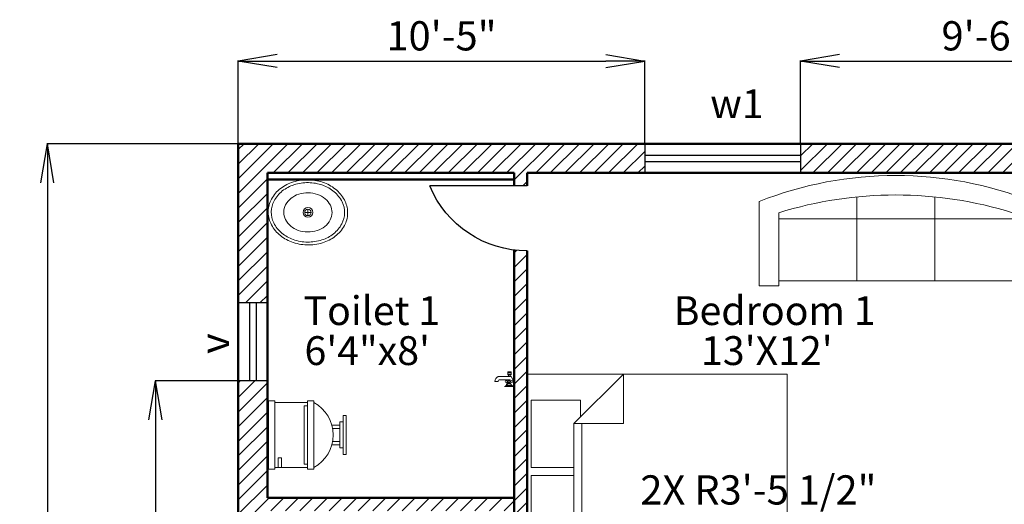
# Model space of a CAD drawing. Units: inches. Extents: x 1856 to 3350, y 1624 to 2224.
# Tile 2 of 7: x 1856 to 2159, y 2016 to 2165. Entities that reach past the tile are written whole.
import ezdxf

# ---------------------------------------------------------------- set-up
doc = ezdxf.new("R2010")
doc.units = ezdxf.units.IN
for name, color, linetype, lineweight in [('A-ANNO-DIMS', 2, 'Continuous', 18), ('A-ANNO-TEXT', 7, 'Continuous', 18), ('A-AREA-IDEN', 7, 'Continuous', 25), ('A-DOOR', 3, 'Continuous', 25), ('A-FLOR-FIXT', 3, 'Continuous', 18), ('A-FURN', 3, 'Continuous', 18), ('A-WALL', 7, 'Continuous', 50), ('A-WALL-PATT', 8, 'Continuous', 13), ('ventilator', 6, 'Continuous', 25), ('window', 4, 'Continuous', 25)]:
    doc.layers.add(name, color=color, linetype=linetype, lineweight=lineweight)
doc.styles.get("Standard").update_dxf_attribs({"font": 'arial.ttf'})
doc.dimstyles.new('ISO-25', dxfattribs={"dimtxt": 9, "dimasz": 12, "dimexe": 0.125, "dimexo": 0.125, "dimgap": 2, "dimtad": 1, "dimtih": 1, "dimtoh": 1, "dimdec": 1, "dimzin": 11, "dimlunit": 4, "dimtxsty": 'Standard', "dimblk": 'OPEN', "dimcen": -0.125, "dimadec": 0, "dimazin": 0, "dimtfac": 1, "dimtdec": 1, "dimtmove": 0, "dimatfit": 3, "dimfxl": 1, "dimarcsym": 0})

# ---------------------------------------------------------------- blocks, each defined once
blk = doc.blocks.new('_Open')
at = {"color": 0, "linetype": 'ByBlock', "lineweight": -2}
for p, q in [((-1, 0.167), (0, 0)), ((-1, -0.167), (0, 0)), ((0, 0), (-1, 0))]:
    blk.add_line(p, q, dxfattribs=at)
blk = doc.blocks.new('*D4')
at = {"layer": 'A-ANNO-DIMS', "color": 0, "lineweight": -2, "transparency": 16777216}
for p, q in [((1922.99, 2126.99), (1864.24, 2126.99)), ((1864.36, 2114.99), (1864.36, 1983.59)), ((1864.36, 1838.99), (1864.36, 1970.4)), ((1922.99, 1826.99), (1864.24, 1826.99))]:
    blk.add_line(p, q, dxfattribs=at)
at = {"layer": 'Defpoints', "color": 0, "transparency": 16777216}
for p in [(1923.11, 2126.99), (1864.36, 1826.99), (1923.11, 1826.99)]:
    blk.add_point(p, dxfattribs=at)
at = {"layer": 'A-ANNO-DIMS', "color": 0, "lineweight": -2, "transparency": 16777216, "xscale": 12, "yscale": 12, "zscale": 12}
for p, rotation in [((1864.36, 2126.99), 90), ((1864.36, 1826.99), 270)]:
    blk.add_blockref('_Open', p, dxfattribs=dict(at, rotation=rotation))
at = {"layer": 'A-ANNO-DIMS', "color": 0, "transparency": 16777216, "insert": (1864.36, 1976.99), "char_height": 9, "attachment_point": 5}
blk.add_mtext("25'", dxfattribs=at)
blk = doc.blocks.new('Sink - Oval top')
for p, q in [((-1, 0), (1, 0)), ((0, 1), (0, -1))]:
    blk.add_line(p, q)
for points in [[(-12.23, 0.39, 0.117634), (-11.46, -3.36, 0.104469), (-8.88, -6.8, 0.090016), (-5.08, -9.07, 0.08192), (-0.32, -10.02, 0.08192), (4.49, -9.38, 0.090016), (8.42, -7.36, 0.104469), (11.22, -4.09, 0.117634), (12.23, -0.39, 0.117634), (11.46, 3.36, 0.104469), (8.88, 6.8, 0.090016), (5.08, 9.07, 0.08192), (0.32, 10.02, 0.08192), (-4.49, 9.38, 0.090016), (-8.42, 7.36, 0.104469), (-11.22, 4.09, 0.117634)], [(-11.29, 0.16, 0.118622), (-10.52, -3.25, 0.104678), (-8.07, -6.36, 0.089562), (-4.54, -8.37, 0.081185), (-0.13, -9.15, 0.081185), (4.3, -8.49, 0.089562), (7.89, -6.58, 0.104678), (10.42, -3.55, 0.118622), (11.29, -0.16, 0.118622), (10.52, 3.25, 0.104678), (8.07, 6.36, 0.089562), (4.54, 8.37, 0.081185), (0.13, 9.15, 0.081185), (-4.3, 8.49, 0.089562), (-7.89, 6.58, 0.104678), (-10.42, 3.55, 0.118622)], [(-7.42, 0.08, 0.118283), (-6.91, -2.17, 0.104607), (-5.29, -4.21, 0.089718), (-2.97, -5.53, 0.081436), (-0.07, -6.04, 0.081436), (2.84, -5.59, 0.089718), (5.2, -4.33, 0.104607), (6.86, -2.32, 0.118283), (7.42, -0.08, 0.118283), (6.91, 2.17, 0.104607), (5.29, 4.21, 0.089718), (2.97, 5.53, 0.081436), (0.07, 6.04, 0.081436), (-2.84, 5.59, 0.089718), (-5.2, 4.33, 0.104607), (-6.86, 2.32, 0.118283)]]:
    blk.add_lwpolyline(points, format="xyb", close=True)
for radius in [1.5, 1]:
    blk.add_circle((0, 0), radius)
blk = doc.blocks.new('Toilet - front')
for p, q in [((-10, 22), (-10, 12)), ((10, 12), (10, 22)), ((-10, 21), (-7, 21)), ((-7, 20), (-10, 20)), ((-7, 21), (-7, 20)), ((9, 13), (-9, 13)), ((-9, 13), (-9, 12)), ((9, 12), (9, 13)), ((10.5, 12), (-10.5, 12)), ((-10.5, 10), (-10.5, 12)), ((10.5, 10), (-10.5, 10)), ((10.5, 12), (10.5, 10)), ((-3, 4.4065), (-3, 2)), ((-2, 2), (-2, 4.1658)), ((2, 4.1658), (2, 2)), ((3, 2), (3, 4.4065)), ((4, 2), (-4, 2)), ((-4, 2), (-4, 1)), ((4, 1), (4, 2))]:
    blk.add_line(p, q)
for points in [[(10.5, 22), (10.5, 24), (-10.5, 24), (-10.5, 22)], [(6, 0), (6, 1), (-6, 1), (-6, 0)]]:
    blk.add_lwpolyline(points, close=True)
blk.add_arc((0, 15.3333), 11.3333, 208.0725, 331.9275)
blk = doc.blocks.new('Bed - Queen')
for p, q in [((0, -80.00003), (0, 0)), ((0, 0), (59.99999, 0)), ((59.99999, 0), (59.99999, -80.00003)), ((7.99999, -1.2), (28.79998, -1.2)), ((7.99999, -14.4), (7.99999, -1.2)), ((28.79998, -1.2), (28.79998, -14.4)), ((31.19999, -1.2), (51.99999, -1.2)), ((31.19999, -14.4), (31.19999, -1.2)), ((51.99999, -1.2), (51.99999, -16.4)), ((0, -14.4), (44.8, -14.4)), ((59.99999, -29.6), (44.8, -14.4)), ((44.8, -14.4), (44.8, -29.6)), ((44.8, -16.8), (0, -16.8)), ((51.99999, -16.4), (46.79936, -16.4)), ((44.8, -29.6), (59.99999, -29.6)), ((59.99999, -80.00003), (0, -80.00003))]:
    blk.add_line(p, q)
blk = doc.blocks.new('Sofa - Roundback 7 ft.')
for p, q in [((-12.00002, -32.4421), (-12.00003, -6.5971)), ((11.99997, -32.4421), (11.99998, -6.5971)), ((-36.000027, -34), (-36.000027, -11.4696)), ((35.99998, -34), (35.99998, -11.4696)), ((-35.999844, -13.3819), (35.9998, -13.3819)), ((-36.000027, -32.4421), (35.99998, -32.4421))]:
    blk.add_line(p, q)
for points in [[(-36.000027, -34), (-42.000027, -34), (-42.000027, -8)], [(41.99998, -8), (41.99998, -34), (35.99998, -34)]]:
    blk.add_lwpolyline(points)
for centre, radius, start, end in [((0, -114.25), 114.25, 68.43141, 111.5686), ((-0.00001, -127.1968), 121.1968, 72.72033, 107.2797)]:
    blk.add_arc(centre, radius, start, end)
blk = doc.blocks.new('Faucet - Bathroom side')
for p, q in [((-0.625, 4.25), (0.375, 4.25)), ((0.375, 3.75), (-0.625, 3.75)), ((-0.375, 3), (-0.375, 3.5)), ((0.125, 3.5), (0.125, 3)), ((-1.625, 0), (-1.375, 0)), ((-1.375, 0), (1.375, 0)), ((-0.88366, 0.25), (0.88424, 0.25)), ((-0.625, 3), (3.375, 3)), ((-0.375, 1.625), (-0.625, 1.625)), ((-0.375, 1.375), (-0.625, 1.375)), ((0.48078, 0.75), (-0.47286, 0.75)), ((2.875, 2), (0.375, 2)), ((0.375, 1.625), (0.625, 1.625)), ((0.375, 1.375), (0.625, 1.375)), ((4.375, 1.5), (3.375, 1.5))]:
    blk.add_line(p, q)
for points in [[(-0.625, 3.75), (-0.625, 4.25)], [(-0.375, 4.5), (0.125, 4.5)], [(0.125, 3.5), (-0.375, 3.5)], [(0.375, 4.25), (0.375, 3.75)]]:
    blk.add_lwpolyline(points)
blk.add_lwpolyline([(-0.375, 1), (-0.375, 2), (0.375, 2), (0.375, 1)], close=True)
for centre in [(-0.875, 1.5), (0, 1.5), (0.875, 1.5)]:
    blk.add_circle(centre, 0.27951)
for centre, radius, start, end in [((-0.38253, 4.2575), 0.24259, 88.22243, 181.7776), ((-0.38253, 3.7424), 0.24259, 178.2224, 271.7776), ((0.13252, 4.2575), 0.24259, 358.2224, 91.77757), ((0.13252, 3.7424), 0.24259, 268.2224, 1.777565), ((3.45929, -0.0281), 5.08436, 143.4467, 179.6834), ((-1.75, 1.375), 1.42522, 285.2551, 344.7449), ((1.75, 1.375), 1.42522, 195.2551, 254.7449), ((-2.49562, -0.286), 3.38273, 9.709485, 29.48735), ((2.96867, 1.5936), 0.41699, 347.0192, 102.9808), ((2.70708, 1.4714), 1.66816, 0.9827695, 66.39737)]:
    blk.add_arc(centre, radius, start, end)
blk = doc.blocks.new('WIN-48')
for p, q in [((0, 9), (48, 9)), ((0, 9), (0, 0)), ((48, 9), (48, 0)), ((0, 5.5), (48, 5.5)), ((0, 3.5), (48, 3.5)), ((0, 0), (48, 0))]:
    blk.add_line(p, q)
blk = doc.blocks.new('VENT-24')
for p, q in [((0, 9), (24, 9)), ((0, 9), (0, 0)), ((24, 9), (24, 0)), ((0, 5.5), (24, 5.5)), ((0, 3.5), (24, 3.5)), ((0, 0), (24, 0))]:
    blk.add_line(p, q)
blk = doc.blocks.new('DOOR-SWING-30')
blk.add_line((30, 0), (0, 0))
blk.add_arc((30, -12.5), 32.5, 90, 157.3801)
blk = doc.blocks.new('*D65')
at = {"layer": 'A-ANNO-DIMS', "color": 0, "lineweight": -2, "transparency": 16777216}
for p, q in [((1923.11, 2127.12), (1923.11, 2152.57)), ((1935.11, 2152.44), (2036.3, 2152.44)), ((2048.3, 2127.12), (2048.3, 2152.57))]:
    blk.add_line(p, q, dxfattribs=at)
at = {"layer": 'Defpoints', "color": 0, "transparency": 16777216}
for p in [(2048.3, 2152.44), (1923.11, 2126.99), (2048.3, 2126.99)]:
    blk.add_point(p, dxfattribs=at)
at = {"layer": 'A-ANNO-DIMS', "color": 0, "lineweight": -2, "transparency": 16777216, "xscale": 12, "yscale": 12, "zscale": 12, "rotation": 180}
blk.add_blockref('_Open', (1923.11, 2152.44), dxfattribs=at)
at = {"layer": 'A-ANNO-DIMS', "color": 0, "lineweight": -2, "transparency": 16777216, "xscale": 12, "yscale": 12, "zscale": 12}
blk.add_blockref('_Open', (2048.3, 2152.44), dxfattribs=at)
at = {"layer": 'A-ANNO-DIMS', "color": 0, "transparency": 16777216, "insert": (1985.71, 2159.04), "char_height": 9, "attachment_point": 5}
blk.add_mtext('10\'-5"', dxfattribs=at)
blk = doc.blocks.new('*D66')
at = {"layer": 'A-ANNO-DIMS', "color": 0, "lineweight": -2, "transparency": 16777216}
for p, q in [((2096.3, 2127.12), (2096.3, 2152.57)), ((2108.3, 2152.44), (2198.14, 2152.44)), ((2210.14, 2127.12), (2210.14, 2152.57))]:
    blk.add_line(p, q, dxfattribs=at)
at = {"layer": 'Defpoints', "color": 0, "transparency": 16777216}
for p in [(2210.14, 2152.44), (2096.3, 2126.99), (2210.14, 2126.99)]:
    blk.add_point(p, dxfattribs=at)
at = {"layer": 'A-ANNO-DIMS', "color": 0, "lineweight": -2, "transparency": 16777216, "xscale": 12, "yscale": 12, "zscale": 12, "rotation": 180}
blk.add_blockref('_Open', (2096.3, 2152.44), dxfattribs=at)
at = {"layer": 'A-ANNO-DIMS', "color": 0, "lineweight": -2, "transparency": 16777216, "xscale": 12, "yscale": 12, "zscale": 12}
blk.add_blockref('_Open', (2210.14, 2152.44), dxfattribs=at)
at = {"layer": 'A-ANNO-DIMS', "color": 0, "transparency": 16777216, "insert": (2153.22, 2159.04), "char_height": 9, "attachment_point": 5}
blk.add_mtext('9\'-6"', dxfattribs=at)
blk = doc.blocks.new('*D72')
at = {"layer": 'A-ANNO-DIMS', "color": 0, "lineweight": -2, "transparency": 16777216}
for p, q in [((1922.99, 2053.99), (1897.54, 2053.99)), ((1897.66, 2041.99), (1897.66, 2004.59)), ((1897.66, 1953.99), (1897.66, 1991.4)), ((1922.99, 1941.99), (1897.54, 1941.99))]:
    blk.add_line(p, q, dxfattribs=at)
at = {"layer": 'Defpoints', "color": 0, "transparency": 16777216}
for p in [(1897.66, 2053.99), (1923.11, 2053.99), (1923.11, 1941.99)]:
    blk.add_point(p, dxfattribs=at)
at = {"layer": 'A-ANNO-DIMS', "color": 0, "lineweight": -2, "transparency": 16777216, "xscale": 12, "yscale": 12, "zscale": 12}
for p, rotation in [((1897.66, 2053.99), 90), ((1897.66, 1941.99), 270)]:
    blk.add_blockref('_Open', p, dxfattribs=dict(at, rotation=rotation))
at = {"layer": 'A-ANNO-DIMS', "color": 0, "transparency": 16777216, "insert": (1897.66, 1997.99), "char_height": 9, "attachment_point": 5}
blk.add_mtext('9\'-4"', dxfattribs=at)
blk = doc.blocks.new('*D91')
at = {"layer": 'A-ANNO-DIMS', "color": 0, "lineweight": -2, "transparency": 16777216}
for p, q in [((2046.79, 2012.59), (2121.79, 2012.59)), ((2121.79, 2012.59), (2132.16, 2005.05)), ((2175.32, 1973.66), (2141.86, 1997.99))]:
    blk.add_line(p, q, dxfattribs=at)
at = {"layer": 'Defpoints', "color": 0, "transparency": 16777216}
for p in [(2141.86, 1997.99), (2175.32, 1973.66)]:
    blk.add_point(p, dxfattribs=at)
at = {"layer": 'A-ANNO-DIMS', "color": 0, "lineweight": -2, "transparency": 16777216, "xscale": 12, "yscale": 12, "zscale": 12, "rotation": 323.9723172818348}
blk.add_blockref('_Open', (2141.86, 1997.99), dxfattribs=at)
at = {"layer": 'A-ANNO-DIMS', "color": 0, "transparency": 16777216, "insert": (2083.29, 2019.25), "char_height": 9, "attachment_point": 5}
blk.add_mtext('2X R3\'-5 1/2"', dxfattribs=at)

msp = doc.modelspace()

# ---------------------------------------------------------------- hatches: boundary and pattern name
at = {"layer": 'A-WALL-PATT'}
h = msp.add_hatch(dxfattribs=at)
h.set_pattern_fill('ANSI31', color=256)
h.paths.add_polyline_path([(2210.14, 2126.99), (2096.3, 2126.99), (2096.3, 2117.99), (2210.14, 2117.99)])
h.paths.add_polyline_path([(2048.3, 2126.99), (1923.11, 2126.99), (1923.11, 2077.99), (1932.11, 2077.99), (1932.11, 2117.99), (2006.11, 2117.99), (2008.11, 2117.99), (2008.11, 2113.99), (2012.11, 2113.99), (2012.11, 2117.99), (2048.29, 2117.99)])
h.paths.add_polyline_path([(2277.11, 2126.99), (2234.14, 2126.99), (2234.14, 2117.99), (2268.11, 2117.99), (2268.11, 1997.99), (2266.11, 1997.99), (2266.11, 1993.99), (2268.11, 1993.99), (2268.11, 1937.99), (2277.11, 1937.99)])
h.paths.add_polyline_path([(2277.11, 1887.99), (2268.11, 1887.99), (2268.11, 1835.99), (2229.11, 1835.99), (2229.11, 1826.99), (2277.11, 1826.99)])
h.paths.add_polyline_path([(2056.11, 1895.99), (2152.11, 1895.99), (2152.11, 1859.99), (2156.11, 1859.99), (2156.11, 1899.99), (2056.11, 1899.99), (2056.11, 1933.99), (2052.11, 1933.99), (2052.11, 1835.99), (2008.11, 1835.99), (2008.11, 1826.99), (2080.11, 1826.99), (2080.11, 1835.99), (2056.11, 1835.99)])
h.paths.add_polyline_path([(2169.11, 1835.99), (2156.11, 1835.99), (2156.11, 1837.99), (2152.11, 1837.99), (2152.11, 1835.99), (2104.11, 1835.99), (2104.11, 1826.99), (2169.11, 1826.99)])
h.paths.add_polyline_path([(1932.11, 1893.99), (1923.11, 1893.99), (1923.11, 1826.99), (1960.11, 1826.99), (1960.11, 1835.99), (1932.11, 1835.99)])
h.paths.add_polyline_path([(1932.11, 2013.99), (2008.11, 2013.99), (2008.11, 2017.99), (1932.11, 2017.99), (1932.11, 2053.99), (1923.11, 2053.99), (1923.11, 1941.99), (1932.11, 1941.99)])
h.paths.add_polyline_path([(2012.11, 2093.99, -0.030857), (2008.11, 2094.24), (2008.11, 1969.99), (2048.11, 1969.99), (2048.12, 1973.99), (2012.11, 1973.99)])
h.paths.add_polyline_path([(2172.11, 2117.99), (2168.11, 2117.99), (2168.11, 1969.99), (2172.11, 1969.99), (2172.11, 1993.99), (2234.11, 1993.99, -0.024205), (2233.95, 1997.99), (2172.11, 1997.99)])
h.paths.add_polyline_path([(2133.95, 1973.99), (2048.12, 1973.99), (2048.11, 1969.99), (2052.11, 1969.99), (2052.11, 1967.99), (2056.11, 1967.99), (2056.11, 1969.99), (2134.11, 1969.99, -0.024205)])

# ---------------------------------------------------------------- linework, layer by layer
at = {"layer": 'A-WALL'}
for p, q in [((1923.11, 2126.99), (2277.11, 2126.99)), ((1923.11, 2126.99), (1923.11, 1826.99)), ((1932.11, 2117.99), (2006.11, 2117.99)), ((1932.11, 2117.99), (1932.11, 2017.99)), ((2006.11, 2117.99), (2008.11, 2117.99)), ((2008.11, 2117.99), (2008.11, 2113.99)), ((2012.11, 2117.99), (2012.11, 2113.99)), ((2012.11, 2117.99), (2268.11, 2117.99)), ((1932.11, 2115.99), (2008.11, 2115.99)), ((2008.11, 2094.24), (2008.11, 2017.99)), ((2008.11, 2093.99), (2008.11, 1969.99)), ((2012.11, 2093.99), (2012.11, 1973.99)), ((2008.11, 2017.99), (1932.11, 2017.99))]:
    msp.add_line(p, q, dxfattribs=at)
at = {"layer": 'ventilator'}
for p, q in [((1932.11, 2077.99), (1923.11, 2077.99)), ((1932.11, 2053.99), (1923.11, 2053.99))]:
    msp.add_line(p, q, dxfattribs=at)
at = {"layer": 'window'}
msp.add_line((2048.3, 2126.99), (2048.29, 2117.99), dxfattribs=at)

# ---------------------------------------------------------------- block references
at = {"layer": 'A-DOOR', "extrusion": (0, 0, -1), "zscale": -1, "rotation": 180}
msp.add_blockref('DOOR-SWING-30', (-1982.11, 2113.99), dxfattribs=at)
at = {"layer": 'A-FLOR-FIXT'}
msp.add_blockref('Sink - Oval top', (1944.59, 2105.86), dxfattribs=at)
at = {"layer": 'A-FLOR-FIXT', "xscale": -1}
msp.add_blockref('Faucet - Bathroom side', (2006.51, 2052.3), dxfattribs=at)
at = {"layer": 'A-FLOR-FIXT', "rotation": 90}
msp.add_blockref('Toilet - front', (1956.41, 2037.33), dxfattribs=at)
at = {"layer": 'A-FURN'}
msp.add_blockref('Sofa - Roundback 7 ft.', (2125.57, 2117.22), dxfattribs=at)
at = {"layer": 'A-FURN', "rotation": 90}
msp.add_blockref('Bed - Queen', (2012.11, 1996.1), dxfattribs=at)
at = {"layer": 'ventilator', "rotation": 269.9999999999983}
msp.add_blockref('VENT-24', (1923.11, 2077.99), dxfattribs=at)
at = {"layer": 'window'}
msp.add_blockref('WIN-48', (2048.3, 2117.99), dxfattribs=at)

# ---------------------------------------------------------------- texts
at = {"layer": 'A-ANNO-TEXT'}
msp.add_text('w1', height=8.871, dxfattribs=at).set_placement((2068.47, 2134.86))
msp.add_text('v', height=8.87, rotation=90, dxfattribs=at).set_placement((1920.32, 2062.31))
at = {"layer": 'A-AREA-IDEN'}
for s, height, p in [('Toilet 1', 8.871, (1943.24, 2071.18)), ('Bedroom 1', 8.871, (2057.2, 2071.18)), (' 6\'4"x8\'', 8.871, (1940.82, 2058.87)), ("    13'X12'", 8.8713, (2054.78, 2058.87))]:
    msp.add_text(s, height=height, dxfattribs=at).set_placement(p)

# ---------------------------------------------------------------- dimensions: what is measured, and where the dimension line sits
at = {"layer": 'A-ANNO-DIMS'}
for base, p1, p2, picture, middle in [((2048.3, 2152.44), (1923.11, 2126.99), (2048.3, 2126.99), '*D65', (1985.71, 2159.04)), ((2210.14, 2152.44), (2096.3, 2126.99), (2210.14, 2126.99), '*D66', (2153.22, 2159.04))]:
    dim = msp.add_linear_dim(base=base, p1=p1, p2=p2, dimstyle='ISO-25', override={"dimdec": 1, "dimlfac": 1, "dimrnd": 0, "dimzin": 1, "dimdsep": 46, "dimlunit": 4, "dimfrac": 2}, dxfattribs=at)
    dim.commit()
    dim.dimension.update_dxf_attribs({"geometry": picture, "text_midpoint": middle})
dim = msp.add_linear_dim(base=(1864.36, 1826.99), p1=(1923.11, 2126.99), p2=(1923.11, 1826.99), angle=90, text="25'", dimstyle='ISO-25', override={"dimclrd": 0, "dimclre": 0, "dimclrt": 0}, dxfattribs=at)
dim.commit()
dim.dimension.update_dxf_attribs({"geometry": '*D4', "text_midpoint": (1864.36, 1976.99)})
dim = msp.add_linear_dim(base=(1897.66, 2053.99), p1=(1923.11, 1941.99), p2=(1923.11, 2053.99), angle=90, dimstyle='ISO-25', override={"dimdec": 1, "dimlfac": 1, "dimrnd": 0, "dimzin": 1, "dimdsep": 46, "dimlunit": 4, "dimfrac": 2}, dxfattribs=at)
dim.commit()
dim.dimension.update_dxf_attribs({"geometry": '*D72', "text_midpoint": (1897.66, 1997.99)})
dim = msp.add_radius_dim(center=(2175.32, 1973.66), mpoint=(2141.86, 1997.99), text='2X <>', dimstyle='ISO-25', override={"dimdec": 1, "dimlfac": 1, "dimrnd": 0, "dimzin": 1, "dimdsep": 46, "dimlunit": 4, "dimfrac": 2}, dxfattribs=at)
dim.commit()
dim.dimension.update_dxf_attribs({"geometry": '*D91', "text_midpoint": (2083.29, 2012.59), "dimtype": 164})

doc.saveas('drawing.dxf')
